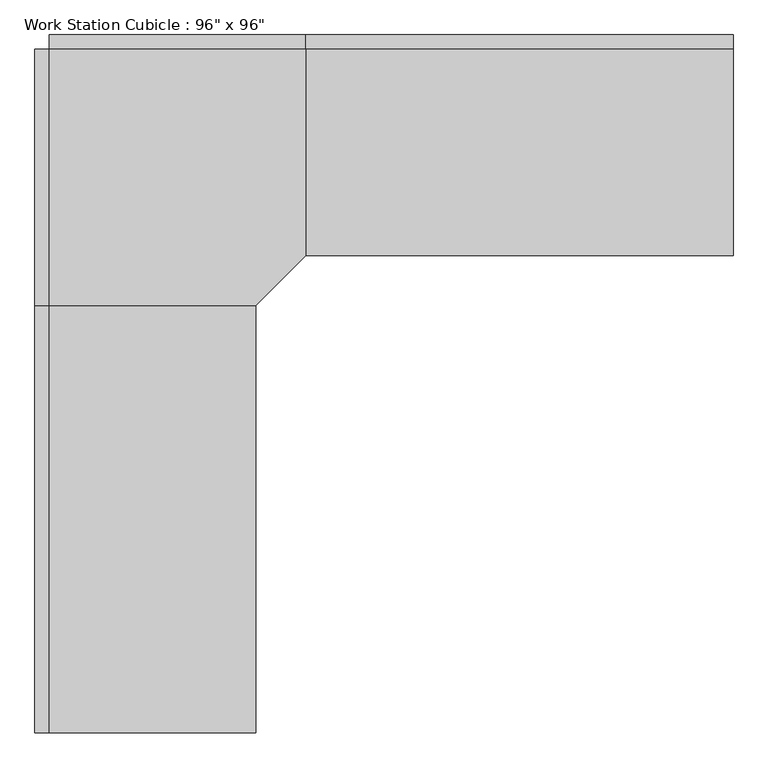
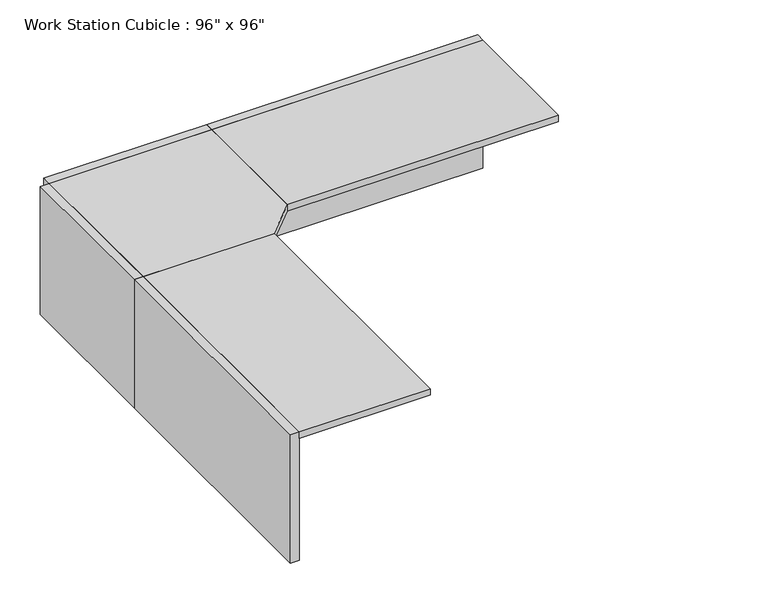
"""IFC4 building model written with IfcOpenShell, lengths in millimetres: furniture geometry."""

from ifc_helpers import new_model, si_unit, frame, origin, origin_with_axes, place, context, project, spatial, polyline, outline, extrude, source, transform, mapped, element, save


def furniture_356da175(model_context):
    return source(origin(), model_context, "Body", "SweptSolid", [
        extrude(outline(polyline([(-80.9317522, -545.8230076), (833.4682478, -545.8230076), (833.4682478, -1282.4230076), (655.6682478, -1460.2230076), (-80.9317522, -1460.2230076), (-80.9317522, -545.8230076)])), frame((0.0, 0.0, 723.9), z_axis=(0.0, 0.0, 1.0), x_axis=(1.0, 0.0, 0.0)), (0.0, 0.0, 1.0), 38.1),
        extrude(outline(polyline([(655.6682478, -2984.2230076), (-80.9317522, -2984.2230076), (-80.9317522, -1460.2230076), (655.6682478, -1460.2230076), (655.6682478, -2984.2230076)])), frame((0.0, 0.0, 723.9), z_axis=(0.0, 0.0, 1.0), x_axis=(1.0, 0.0, 0.0)), (0.0, 0.0, 1.0), 38.1),
        extrude(outline(polyline([(2357.4682478, -1282.4230076), (833.4682478, -1282.4230076), (833.4682478, -545.8230076), (2357.4682478, -545.8230076), (2357.4682478, -1282.4230076)])), frame((0.0, 0.0, 723.9), z_axis=(0.0, 0.0, 1.0), x_axis=(1.0, 0.0, 0.0)), (0.0, 0.0, 1.0), 38.1),
        extrude(outline(polyline([(2357.4682478, -545.8230076), (833.4682478, -545.8230076), (833.4682478, -495.0230076), (2357.4682478, -495.0230076), (2357.4682478, -545.8230076)])), origin_with_axes(), (0.0, 0.0, 1.0), 762.0),
        extrude(outline(polyline([(833.4682478, -545.8230076), (-80.9317522, -545.8230076), (-80.9317522, -495.0230076), (833.4682478, -495.0230076), (833.4682478, -545.8230076)])), origin_with_axes(), (0.0, 0.0, 1.0), 762.0),
        extrude(outline(polyline([(-80.9317522, -1460.2230076), (-131.7317522, -1460.2230076), (-131.7317522, -545.8230076), (-80.9317522, -545.8230076), (-80.9317522, -1460.2230076)])), origin_with_axes(), (0.0, 0.0, 1.0), 762.0),
        extrude(outline(polyline([(-80.9317522, -2984.2230076), (-131.7317522, -2984.2230076), (-131.7317522, -1460.2230076), (-80.9317522, -1460.2230076), (-80.9317522, -2984.2230076)])), origin_with_axes(), (0.0, 0.0, 1.0), 762.0),
    ])


if __name__ == "__main__":
    model = new_model("IFC4")
    model_context = context("Model", 3, world=origin())
    ifc_project = project(units=[si_unit("LENGTHUNIT", "METRE", prefix="MILLI")], contexts=[model_context])
    site = spatial("IfcSite", under=ifc_project)
    building = spatial("IfcBuilding", under=site)
    placement = place(None, origin())
    furniture_shape = furniture_356da175(model_context)
    element("IfcFurniture", 1, ObjectType="Work Station Cubicle : 96\" x 96\"", at=placement, inside=building, context=model_context, shape_type="MappedRepresentation", body=[
        mapped(furniture_shape, transform((0.0, 0.0, 0.0), x_axis=(1.0, 0.0, 0.0), y_axis=(0.0, 1.0, 0.0), z_axis=(0.0, 0.0, 1.0))),
    ])
    save(model, "model.ifc")

# Revit data of these elements
# Type "Work Station Cubicle : 96\" x 96\""
#   Assembly Code = "E2020"
#   Desktop Height = 2' - 6"
#   Desktop1 Width = 2' - 5"
#   Desktop2 Width = 2' - 5"
#   Panel Height = 2' - 6"
#   Panel1 Length = 5' - 0"
#   Panel2 Length = 5' - 0"
#   Cube Panel Material = Textile - Light Gray
#   Work Top Material = Laminate, Ivory, Matte
#   Default Elevation = 0
# Element 1 (IfcFurniture, "Work Station Cubicle : 96\" x 96\"")
#   Materials on its faces: "Textile - Light Gray", "Laminate, Ivory, Matte"
# Materials
#   "Textile - Light Gray": class "Fabric", colour RGB 204 204 204, transparency 0
#   "Laminate, Ivory, Matte": class "Plastic", colour RGB 247 247 239, transparency 0, Description = "Plastic Laminate - Ivory, Matte", Cost = 0
